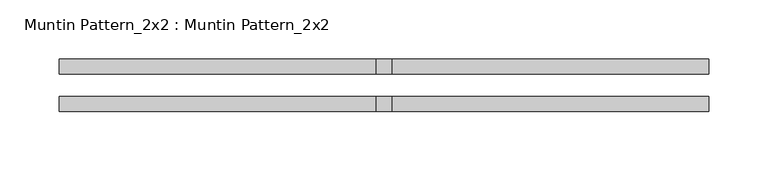
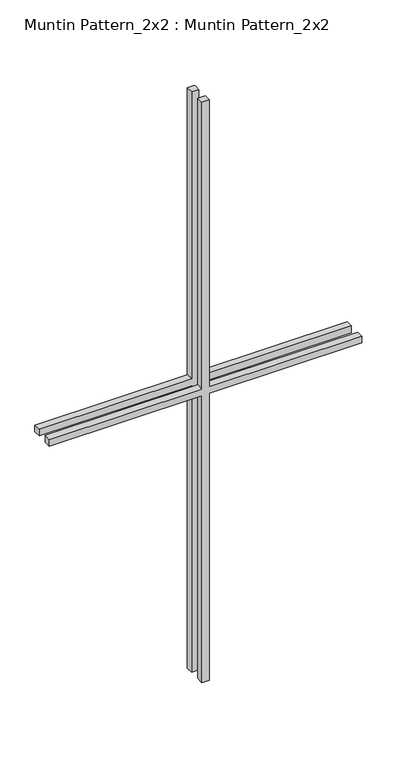
"""IFC4 building model written with IfcOpenShell, lengths in millimetres: proxy geometry, Muntin Pattern_2x2 : Muntin Pattern_2x2."""

from ifc_helpers import new_model, si_unit, frame, origin, place, context, project, spatial, polyline, outline, extrude, source, transform, mapped, element, save


def muntin_pattern_2x2_muntin_pattern_2x2_cdb221ef(model_context):
    return source(origin(), model_context, "Body", "SweptSolid", [
        extrude(outline(polyline([(546.1, -6.35), (546.1, -274.6375), (533.4, -274.6375), (533.4, -6.35), (0.0, -6.35), (0.0, 6.35), (533.4, 6.35), (533.4, 274.6375), (546.1, 274.6375), (546.1, 6.35), (1079.5, 6.35), (1079.5, -6.35), (546.1, -6.35)])), frame((0.0, 9.525, 0.0), z_axis=(0.0, 1.0, 0.0), x_axis=(0.0, 0.0, 1.0)), (0.0, 0.0, 1.0), 12.7),
        extrude(outline(polyline([(546.1, -6.35), (546.1, -274.6375), (533.4, -274.6375), (533.4, -6.35), (0.0, -6.35), (0.0, 6.35), (533.4, 6.35), (533.4, 274.6375), (546.1, 274.6375), (546.1, 6.35), (1079.5, 6.35), (1079.5, -6.35), (546.1, -6.35)])), frame((0.0, -22.225, 0.0), z_axis=(0.0, 1.0, 0.0), x_axis=(0.0, 0.0, 1.0)), (0.0, 0.0, 1.0), 12.7),
    ])


if __name__ == "__main__":
    model = new_model("IFC4")
    model_context = context("Model", 3, world=origin())
    ifc_project = project(units=[si_unit("LENGTHUNIT", "METRE", prefix="MILLI")], contexts=[model_context])
    site = spatial("IfcSite", under=ifc_project)
    building = spatial("IfcBuilding", under=site)
    placement = place(None, origin())
    muntin_pattern_2x2_muntin_pattern_2x2_shape = muntin_pattern_2x2_muntin_pattern_2x2_cdb221ef(model_context)
    element("IfcBuildingElementProxy", 1, Name="Muntin Pattern_2x2 : Muntin Pattern_2x2", ObjectType="Muntin Pattern_2x2 : Muntin Pattern_2x2", at=placement, inside=building, context=model_context, shape_type="MappedRepresentation", body=[
        mapped(muntin_pattern_2x2_muntin_pattern_2x2_shape, transform((0.0, 0.0, 0.0), x_axis=(1.0, 0.0, 0.0), y_axis=(0.0, 1.0, 0.0), z_axis=(0.0, 0.0, 1.0))),
    ])
    save(model, "model.ifc")

# Revit data of these elements
# Type "Muntin Pattern_2x2 : Muntin Pattern_2x2"
#   Width [instance default] = 4' - 0"
#   Thickness = 0' - 0 1/2"
#   Height [instance default] = 4' - 0"
#   Distance = 0' - 0 3/4"
#   Interior Material [instance default] = none
#   Exterior Material [instance default] = none
#   Default Elevation = 0
# Element 1 (IfcBuildingElementProxy, "Muntin Pattern_2x2 : Muntin Pattern_2x2")
#   Width = 1' - 9 5/8"
#   Height = 3' - 6 1/2"
#   Interior Material = Wood - Stained
#   Exterior Material = Clad - White
#   Materials on its faces: "Clad - White", "Wood - Stained"
# Materials
#   "Clad - White": class "Wood", colour RGB 242 242 238, transparency 0, Cost = 0
#   "Wood - Stained": class "Wood", colour RGB 224 178 126, transparency 0, Cost = 0
